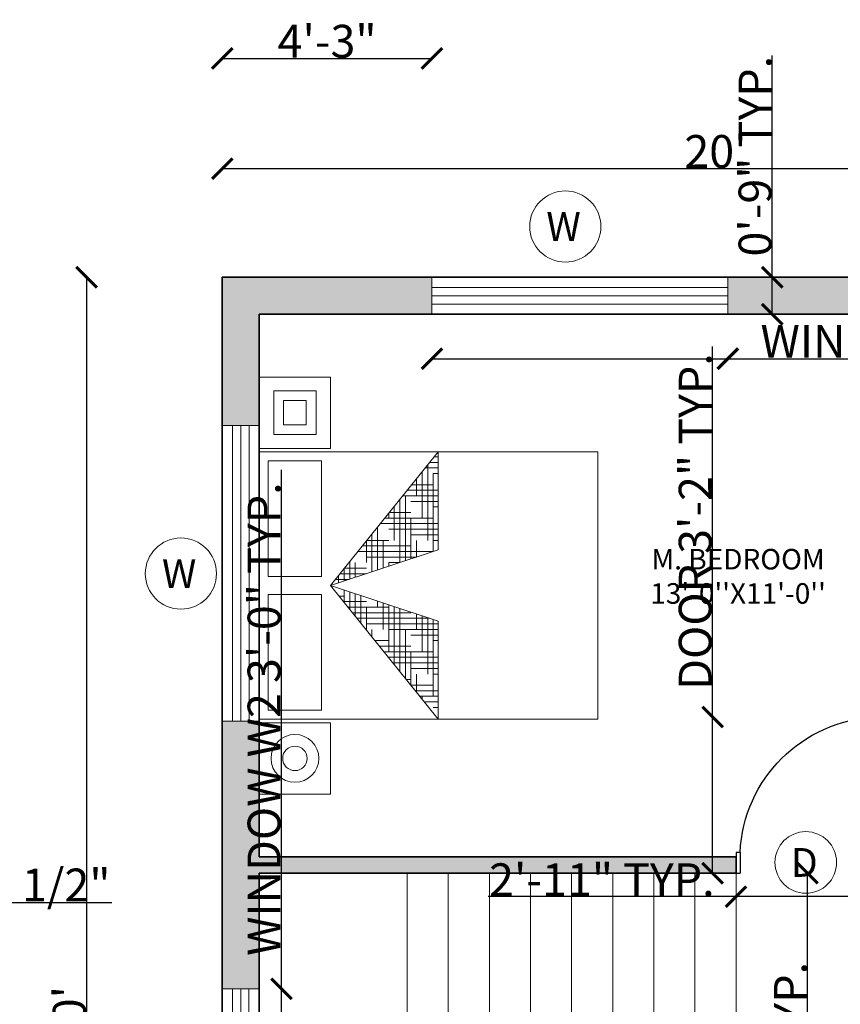
# Model space of a CAD drawing. Units: inches. Extents: x 2209 to 2954, y 1760 to 2265.
# Tile 6 of 7: x 2580 to 2780, y 2005 to 2245. Entities that reach past the tile are written whole.
import ezdxf

# ---------------------------------------------------------------- set-up
doc = ezdxf.new("R2010")
doc.units = ezdxf.units.IN
for name, color, linetype, lineweight in [('A-ANNO-DIMS', 2, 'Continuous', 18), ('A-ANNO-SYMB', 7, 'Continuous', 18), ('A-AREA-IDEN', 7, 'Continuous', 18), ('A-FURN', 8, 'Continuous', 18), ('A-WALL-PATT', 30, 'Continuous', 13), ('DOOR', 240, 'Continuous', 25), ('STEPS', 50, 'Continuous', 18), ('WALL', 7, 'Continuous', 35), ('WINDOW', 190, 'Continuous', 18)]:
    doc.layers.add(name, color=color, linetype=linetype, lineweight=lineweight)
doc.styles.get("Standard").update_dxf_attribs({"font": 'arial.ttf'})
doc.dimstyles.get("Standard").update_dxf_attribs({"dimtxt": 8, "dimasz": 5, "dimexe": 0.18, "dimexo": 0.0625, "dimgap": 0.09, "dimtad": 1, "dimdec": 1, "dimzin": 0, "dimdsep": 46, "dimlunit": 4, "dimtxsty": 'Standard', "dimblk": 'ARCHTICK', "dimcen": 0.09, "dimse1": 1, "dimse2": 1, "dimadec": 0, "dimazin": 0, "dimtfac": 1, "dimtdec": 1, "dimtofl": 0, "dimtmove": 0, "dimatfit": 3, "dimfxl": 1, "dimtolj": 1, "dimtzin": 0, "dimarcsym": 0})

# ---------------------------------------------------------------- blocks, each defined once
blk = doc.blocks.new('AP0B05')
for p, q in [((35, 100), (35, 880)), ((75, 100), (75, 878.9)), ((35, 100), (11, 100)), ((11, 100), (11, -20)), ((35, 100), (35, -20)), ((815, 100), (815, -20)), ((815, 100), (839, 100)), ((839, 100), (839, -20)), ((11, -20), (35, -20)), ((839, -20), (815, -20))]:
    blk.add_line(p, q)
blk.add_lwpolyline([(35, 100), (75, 100)])
blk.add_arc((-2.4, 62.6), 818.3, 2.6212, 87.3788)
blk = doc.blocks.new('*X3')
at = {"color": 0}
for p, q in [((20.25, 14.8125), (20.2772, 14.8125)), ((20.1875, 14.75), (20.1875, 14.7669)), ((20.199, 14.7812), (20.2772, 14.7812)), ((20.1487, 14.7188), (20.2772, 14.7188)), ((20.1562, 14.625), (20.1562, 14.7281)), ((20.1739, 14.75), (20.2772, 14.75)), ((20.25, 14.3194), (20.25, 14.75)), ((20.0938, 14.375), (20.0938, 14.6504)), ((20.0984, 14.6562), (20.125, 14.6562)), ((20.1236, 14.6875), (20.25, 14.6875)), ((20.125, 14.5), (20.125, 14.6893)), ((20.0625, 14.2573), (20.0625, 14.6116)), ((20.125, 14.5938), (20.2772, 14.5938)), ((20.2188, 14.3091), (20.2188, 14.625)), ((20.25, 14.625), (20.2772, 14.625)), ((20.023, 14.5625), (20.2772, 14.5625)), ((20.0312, 14.2469), (20.0312, 14.5727)), ((19.9727, 14.5), (20.25, 14.5)), ((19.9979, 14.5312), (20.2772, 14.5312)), ((20, 14.2366), (20, 14.5)), ((20.1875, 14.2987), (20.1875, 14.5)), ((19.9225, 14.4375), (20, 14.4375)), ((19.9476, 14.4688), (20.125, 14.4688)), ((20.25, 14.4375), (20.2772, 14.4375)), ((19.875, 14.25), (19.875, 14.3785)), ((19.9062, 14.375), (19.9062, 14.4174)), ((19.9688, 14.2262), (19.9688, 14.375)), ((20, 14.375), (20.2772, 14.375)), ((20.125, 14.4062), (20.2772, 14.4062)), ((20.1562, 14.2884), (20.1562, 14.375)), ((19.8219, 14.3125), (20.2291, 14.3125)), ((19.8438, 14.1848), (19.8438, 14.3397)), ((19.875, 14.3438), (20.2772, 14.3438)), ((19.7812, 14.1641), (19.7812, 14.262)), ((19.7967, 14.2812), (20.125, 14.2812)), ((19.8125, 14.1744), (19.8125, 14.3008)), ((19.7465, 14.2188), (19.875, 14.2188)), ((19.75, 14.1537), (19.75, 14.2231)), ((19.7716, 14.25), (20, 14.25)), ((19.9375, 14.2159), (19.9375, 14.25)), ((19.7213, 14.1875), (19.75, 14.1875)), ((19.7018, 14.0938), (19.7786, 14.0938)), ((19.7188, 14.0726), (19.7188, 14.1136)), ((19.75, 14.0338), (19.75, 14.1032)), ((19.7812, 13.9949), (19.7812, 14.0929)), ((19.7269, 14.0625), (19.8728, 14.0625)), ((19.8125, 14), (19.8125, 14.0825)), ((19.9062, 13.8396), (19.9062, 14.0514)), ((19.9375, 13.8007), (19.9375, 14.0411)), ((19.752, 14.0312), (19.875, 14.0312)), ((19.875, 13.8784), (19.875, 14)), ((19.9688, 13.875), (19.9688, 14.0307)), ((20, 14), (20, 14.0204)), ((20, 14), (20.0614, 14)), ((20.0625, 13.6454), (20.0625, 13.9996)), ((20.0938, 13.625), (20.0938, 13.9893)), ((19.8275, 13.9375), (20.25, 13.9375)), ((19.875, 13.9688), (20.1557, 13.9688)), ((20.125, 13.75), (20.125, 13.9789)), ((20.1562, 13.875), (20.1562, 13.9686)), ((20.25, 13.5), (20.25, 13.9375)), ((19.8526, 13.9062), (20.125, 13.9062)), ((19.8777, 13.875), (20, 13.875)), ((20.0312, 13.6842), (20.0312, 13.875)), ((20.2188, 13.4511), (20.2188, 13.875)), ((20.25, 13.875), (20.2772, 13.875)), ((20.125, 13.8438), (20.2772, 13.8438)), ((19.9532, 13.7812), (20.2772, 13.7812)), ((20, 13.8125), (20.2772, 13.8125)), ((19.9783, 13.75), (20.25, 13.75)), ((20, 13.723), (20, 13.75)), ((20.0035, 13.7188), (20.125, 13.7188)), ((20.1875, 13.49), (20.1875, 13.75)), ((20.125, 13.6562), (20.2772, 13.6562)), ((20.25, 13.6875), (20.2772, 13.6875)), ((20.0789, 13.625), (20.2772, 13.625)), ((20.104, 13.5938), (20.2772, 13.5938)), ((20.1562, 13.5288), (20.1562, 13.625)), ((20.1292, 13.5625), (20.25, 13.5625)), ((20.25, 13.5), (20.2772, 13.5)), ((20.2046, 13.4688), (20.2772, 13.4688)), ((20.2297, 13.4375), (20.2772, 13.4375)), ((20.2549, 13.4062), (20.2772, 13.4062))]:
    blk.add_line(p, q, dxfattribs=at)
blk = doc.blocks.new('MAT-P13')
for p, q in [((-1.17, 0), (-1.17, -0.4)), ((-1.17, 0), (-0.77, 0)), ((-0.77, 0), (-0.77, -0.4)), ((-0.75, 0), (0.75, 0)), ((-0.75, 0), (-0.75, -1.9)), ((0.75, 0), (0.75, -1.9)), ((0.77, 0), (1.17, 0)), ((0.77, 0), (0.77, -0.4)), ((1.17, 0), (1.17, -0.4)), ((-0.7, -0.05), (-0.7, -0.35)), ((-0.7, -0.05), (-0.05, -0.05)), ((-0.05, -0.35), (-0.05, -0.05)), ((0.05, -0.05), (0.7, -0.05)), ((0.05, -0.35), (0.05, -0.05)), ((0.7, -0.05), (0.7, -0.35)), ((-0.7, -0.35), (-0.05, -0.35)), ((0.05, -0.35), (0.7, -0.35)), ((-1.17, -0.4), (-0.77, -0.4)), ((-0.75, -1.0034), (0, -0.4)), ((0, -0.4), (-0.75, -1.0034)), ((0, -0.4), (-0.2, -1.0034)), ((0, -0.4), (0.2, -1.0034)), ((0, -0.4), (0.75, -1.0034)), ((0.77, -0.4), (1.17, -0.4)), ((-0.75, -1.0034), (-0.2, -1.0034)), ((0.2, -1.0034), (0.75, -1.0034)), ((0.75, -1.9), (-0.75, -1.9))]:
    blk.add_line(p, q)
for points in [[(0.8468, -0.0814), (1.0932, -0.0814), (1.0932, -0.3186), (0.8468, -0.3186)], [(0.9015, -0.1361), (1.0385, -0.1361), (1.0385, -0.2639), (0.9015, -0.2639)]]:
    blk.add_lwpolyline(points, close=True)
for radius in [0.1342, 0.0686]:
    blk.add_circle((-0.97, -0.2), radius)
at = {"xscale": -1, "rotation": 90}
blk.add_blockref('*X3', (14.1285, 19.2738), dxfattribs=at)
blk = doc.blocks.new('_ArchTick')
at = {"color": 0, "linetype": 'ByBlock', "const_width": 0.15}
blk.add_lwpolyline([(-0.5, -0.5), (0.5, 0.5)], dxfattribs=at)
blk = doc.blocks.new('*D15')
at = {"layer": 'A-ANNO-DIMS', "color": 0, "lineweight": -2, "transparency": 16777216}
blk.add_line((2629.22, 2208.74), (2869.22, 2208.74), dxfattribs=at)
at = {"layer": 'Defpoints', "color": 0, "transparency": 16777216}
for p in [(2869.22, 2208.74), (2629.22, 2182.29), (2869.22, 2182.29)]:
    blk.add_point(p, dxfattribs=at)
at = {"layer": 'A-ANNO-DIMS', "color": 0, "lineweight": -2, "transparency": 16777216, "xscale": 5, "yscale": 5, "zscale": 5, "rotation": 180}
blk.add_blockref('_ArchTick', (2629.22, 2208.74), dxfattribs=at)
at = {"layer": 'A-ANNO-DIMS', "color": 0, "lineweight": -2, "transparency": 16777216, "xscale": 5, "yscale": 5, "zscale": 5}
blk.add_blockref('_ArchTick', (2869.22, 2208.74), dxfattribs=at)
at = {"layer": 'A-ANNO-DIMS', "color": 0, "transparency": 16777216, "insert": (2749.22, 2212.91), "char_height": 8, "attachment_point": 5}
blk.add_mtext("\\A1;20'", dxfattribs=at)
blk = doc.blocks.new('*D16')
at = {"layer": 'A-ANNO-DIMS', "color": 0, "lineweight": -2, "transparency": 16777216}
blk.add_line((2596.18, 2182.29), (2596.18, 1822.29), dxfattribs=at)
at = {"layer": 'Defpoints', "color": 0, "transparency": 16777216}
for p in [(2629.22, 2182.29), (2596.18, 1822.29), (2629.22, 1822.29)]:
    blk.add_point(p, dxfattribs=at)
at = {"layer": 'A-ANNO-DIMS', "color": 0, "lineweight": -2, "transparency": 16777216, "xscale": 5, "yscale": 5, "zscale": 5}
for p, rotation in [((2596.18, 2182.29), 90), ((2596.18, 1822.29), 270)]:
    blk.add_blockref('_ArchTick', p, dxfattribs=dict(at, rotation=rotation))
at = {"layer": 'A-ANNO-DIMS', "color": 0, "transparency": 16777216, "insert": (2592, 2002.29), "char_height": 8, "attachment_point": 5, "rotation": 90}
blk.add_mtext("\\A1;30'", dxfattribs=at)
blk = doc.blocks.new('WIN-W-72IN')
for p, q in [((0, 6.5), (72, 6.5)), ((0, 4.5), (72, 4.5)), ((0, 2.5), (72, 2.5))]:
    blk.add_line(p, q)
blk.add_lwpolyline([(0, 9), (72, 9), (72, 0), (0, 0)], close=True)
blk = doc.blocks.new('WIN-W2-36IN')
for p, q in [((2.5, 0), (2.5, 36)), ((4.5, 0), (4.5, 36)), ((6.5, 0), (6.5, 36))]:
    blk.add_line(p, q)
blk.add_lwpolyline([(0, 0), (0, 36), (9, 36), (9, 0)], close=True)
blk = doc.blocks.new('STAIR-RETURN-36IN')
for p, q in [((36, 0), (36, 92)), ((46, 56), (46, 92)), ((56, 56), (56, 92)), ((66, 56), (66, 92)), ((76, 56), (76, 92)), ((86, 56), (86, 92)), ((96, 56), (96, 92)), ((106, 56), (106, 92)), ((116, 56), (116, 92)), ((116, 56), (0, 56)), ((36, 46), (0, 46)), ((106, 36), (0, 36)), ((46, 0), (46, 36)), ((56, 0), (56, 36)), ((66, 0), (66, 36)), ((76, 0), (76, 36)), ((86, 0), (86, 36)), ((96, 0), (96, 36)), ((106, 0), (106, 36))]:
    blk.add_line(p, q)
blk = doc.blocks.new('TAG-OPENING-W')
blk.add_circle((0, 0), 8.66)
blk.add_text('W', height=7).set_placement((-4.62, -3.5))
blk = doc.blocks.new('TAG-OPENING-D')
blk.add_circle((0, 0), 7.5)
blk.add_text('D', height=7).set_placement((-3.65, -3.5))
blk = doc.blocks.new('*D27')
at = {"layer": 'A-ANNO-DIMS', "color": 0, "lineweight": -2, "transparency": 16777216}
for p, q in [((2680.22, 2162.49), (2752.22, 2162.49)), ((2752.22, 2162.49), (2872.28, 2162.49))]:
    blk.add_line(p, q, dxfattribs=at)
at = {"layer": 'Defpoints', "color": 0, "transparency": 16777216}
for p in [(2680.22, 2173.29), (2752.22, 2173.29), (2752.22, 2162.49)]:
    blk.add_point(p, dxfattribs=at)
at = {"layer": 'A-ANNO-DIMS', "color": 0, "lineweight": -2, "transparency": 16777216, "xscale": 5, "yscale": 5, "zscale": 5, "rotation": 180}
blk.add_blockref('_ArchTick', (2680.22, 2162.49), dxfattribs=at)
at = {"layer": 'A-ANNO-DIMS', "color": 0, "lineweight": -2, "transparency": 16777216, "xscale": 5, "yscale": 5, "zscale": 5}
blk.add_blockref('_ArchTick', (2752.22, 2162.49), dxfattribs=at)
at = {"layer": 'A-ANNO-DIMS', "color": 0, "transparency": 16777216, "insert": (2814.75, 2166.71), "char_height": 8, "attachment_point": 5}
blk.add_mtext('\\A1;WINDOW W 6\'-0" TYP.', dxfattribs=at)
blk = doc.blocks.new('*D28')
at = {"layer": 'A-ANNO-DIMS', "color": 0, "lineweight": -2, "transparency": 16777216}
for p, q in [((2763.02, 2182.29), (2763.02, 2236.23)), ((2763.02, 2173.29), (2763.02, 2182.29))]:
    blk.add_line(p, q, dxfattribs=at)
at = {"layer": 'Defpoints', "color": 0, "transparency": 16777216}
for p in [(2752.22, 2182.29), (2763.02, 2182.29), (2752.22, 2173.29)]:
    blk.add_point(p, dxfattribs=at)
at = {"layer": 'A-ANNO-DIMS', "color": 0, "lineweight": -2, "transparency": 16777216, "xscale": 5, "yscale": 5, "zscale": 5}
for p, rotation in [((2763.02, 2182.29), 90), ((2763.02, 2173.29), 270)]:
    blk.add_blockref('_ArchTick', p, dxfattribs=dict(at, rotation=rotation))
at = {"layer": 'A-ANNO-DIMS', "color": 0, "transparency": 16777216, "insert": (2758.84, 2211.76), "char_height": 8, "attachment_point": 5, "rotation": 90}
blk.add_mtext('\\A1;0\'-9" TYP.', dxfattribs=at)
blk = doc.blocks.new('*D29')
at = {"layer": 'A-ANNO-DIMS', "color": 0, "lineweight": -2, "transparency": 16777216}
for p, q in [((2643.62, 2009.14), (2643.62, 2135.42)), ((2643.62, 1973.14), (2643.62, 2009.14))]:
    blk.add_line(p, q, dxfattribs=at)
at = {"layer": 'Defpoints', "color": 0, "transparency": 16777216}
for p in [(2638.22, 2009.14), (2643.62, 2009.14), (2638.22, 1973.14)]:
    blk.add_point(p, dxfattribs=at)
at = {"layer": 'A-ANNO-DIMS', "color": 0, "lineweight": -2, "transparency": 16777216, "xscale": 5, "yscale": 5, "zscale": 5}
for p, rotation in [((2643.62, 2009.14), 90), ((2643.62, 1973.14), 270)]:
    blk.add_blockref('_ArchTick', p, dxfattribs=dict(at, rotation=rotation))
at = {"layer": 'A-ANNO-DIMS', "color": 0, "transparency": 16777216, "insert": (2639.38, 2074.78), "char_height": 8, "attachment_point": 5, "rotation": 90}
blk.add_mtext('\\A1;WINDOW W2 3\'-0" TYP.', dxfattribs=at)
blk = doc.blocks.new('*D37')
at = {"layer": 'A-ANNO-DIMS', "color": 0, "lineweight": -2, "transparency": 16777216}
for p, q in [((2748.52, 2075.28), (2748.52, 2165.46)), ((2748.52, 2037.29), (2748.52, 2075.28))]:
    blk.add_line(p, q, dxfattribs=at)
at = {"layer": 'Defpoints', "color": 0, "transparency": 16777216}
for p in [(2748.52, 2075.28), (2754.22, 2075.28), (2754.22, 2037.29)]:
    blk.add_point(p, dxfattribs=at)
at = {"layer": 'A-ANNO-DIMS', "color": 0, "lineweight": -2, "transparency": 16777216, "xscale": 5, "yscale": 5, "zscale": 5}
for p, rotation in [((2748.52, 2075.28), 90), ((2748.52, 2037.29), 270)]:
    blk.add_blockref('_ArchTick', p, dxfattribs=dict(at, rotation=rotation))
at = {"layer": 'A-ANNO-DIMS', "color": 0, "transparency": 16777216, "insert": (2744.28, 2122.87), "char_height": 8, "attachment_point": 5, "rotation": 90}
blk.add_mtext('\\A1;DOOR 3\'-2" TYP.', dxfattribs=at)
blk = doc.blocks.new('*D38')
at = {"layer": 'A-ANNO-DIMS', "color": 0, "lineweight": -2, "transparency": 16777216}
for p, q in [((2754.22, 2031.59), (2693.92, 2031.59)), ((2789.17, 2031.59), (2754.22, 2031.59))]:
    blk.add_line(p, q, dxfattribs=at)
at = {"layer": 'Defpoints', "color": 0, "transparency": 16777216}
for p in [(2754.22, 2037.29), (2789.17, 2037.29), (2754.22, 2031.59)]:
    blk.add_point(p, dxfattribs=at)
at = {"layer": 'A-ANNO-DIMS', "color": 0, "lineweight": -2, "transparency": 16777216, "xscale": 5, "yscale": 5, "zscale": 5, "rotation": 180}
blk.add_blockref('_ArchTick', (2754.22, 2031.59), dxfattribs=at)
at = {"layer": 'A-ANNO-DIMS', "color": 0, "lineweight": -2, "transparency": 16777216, "xscale": 5, "yscale": 5, "zscale": 5}
blk.add_blockref('_ArchTick', (2789.17, 2031.59), dxfattribs=at)
at = {"layer": 'A-ANNO-DIMS', "color": 0, "transparency": 16777216, "insert": (2721.57, 2035.7), "char_height": 8, "attachment_point": 5}
blk.add_mtext('\\A1;2\'-11" TYP.', dxfattribs=at)
blk = doc.blocks.new('*D52')
at = {"layer": 'A-ANNO-DIMS', "color": 0, "lineweight": -2, "transparency": 16777216}
blk.add_line((2771.62, 1945.29), (2771.62, 2037.29), dxfattribs=at)
at = {"layer": 'Defpoints', "color": 0, "transparency": 16777216}
for p in [(2754.22, 2037.29), (2771.62, 2037.29), (2754.22, 1945.29)]:
    blk.add_point(p, dxfattribs=at)
at = {"layer": 'A-ANNO-DIMS', "color": 0, "lineweight": -2, "transparency": 16777216, "xscale": 5, "yscale": 5, "zscale": 5}
for p, rotation in [((2771.62, 2037.29), 90), ((2771.62, 1945.29), 270)]:
    blk.add_blockref('_ArchTick', p, dxfattribs=dict(at, rotation=rotation))
at = {"layer": 'A-ANNO-DIMS', "color": 0, "transparency": 16777216, "insert": (2767.44, 1991.29), "char_height": 8, "attachment_point": 5, "rotation": 90}
blk.add_mtext('\\A1;7\'-8" TYP.', dxfattribs=at)
blk = doc.blocks.new('*D61')
at = {"layer": 'A-ANNO-DIMS', "color": 0, "lineweight": -2, "transparency": 16777216}
for p, q in [((2429.48, 2030.19), (2506.77, 2030.19)), ((2506.77, 2030.19), (2602.37, 2030.19))]:
    blk.add_line(p, q, dxfattribs=at)
at = {"layer": 'Defpoints', "color": 0, "transparency": 16777216}
for p in [(2506.77, 2030.19), (2429.48, 2018.6), (2506.77, 2018.6)]:
    blk.add_point(p, dxfattribs=at)
at = {"layer": 'A-ANNO-DIMS', "color": 0, "lineweight": -2, "transparency": 16777216, "xscale": 5, "yscale": 5, "zscale": 5, "rotation": 180}
blk.add_blockref('_ArchTick', (2429.48, 2030.19), dxfattribs=at)
at = {"layer": 'A-ANNO-DIMS', "color": 0, "lineweight": -2, "transparency": 16777216, "xscale": 5, "yscale": 5, "zscale": 5}
blk.add_blockref('_ArchTick', (2506.77, 2030.19), dxfattribs=at)
at = {"layer": 'A-ANNO-DIMS', "color": 0, "transparency": 16777216, "insert": (2557.07, 2034.42), "char_height": 8, "attachment_point": 5}
blk.add_mtext('\\A1;DINETTE 6\'-5 1/2"', dxfattribs=at)
blk = doc.blocks.new('*D76')
at = {"layer": 'A-ANNO-DIMS', "color": 0, "lineweight": -2, "transparency": 16777216}
for p, q in [((2920.04, 2077.63), (2920.04, 2129.07)), ((2920.04, 2043.25), (2920.04, 2077.63))]:
    blk.add_line(p, q, dxfattribs=at)
at = {"layer": 'Defpoints', "color": 0, "transparency": 16777216}
for p in [(2519.15, 2077.63), (2920.04, 2077.63), (2519.15, 2043.25)]:
    blk.add_point(p, dxfattribs=at)
at = {"layer": 'A-ANNO-DIMS', "color": 0, "lineweight": -2, "transparency": 16777216, "xscale": 5, "yscale": 5, "zscale": 5}
for p, rotation in [((2920.04, 2077.63), 90), ((2920.04, 2043.25), 270)]:
    blk.add_blockref('_ArchTick', p, dxfattribs=dict(at, rotation=rotation))
at = {"layer": 'A-ANNO-DIMS', "color": 0, "transparency": 16777216, "insert": (2915.82, 2105.85), "char_height": 8, "attachment_point": 5, "rotation": 90}
blk.add_mtext('\\A1;2\'-10 1/2"', dxfattribs=at)
blk = doc.blocks.new('*D77')
at = {"layer": 'A-ANNO-DIMS', "color": 0, "lineweight": -2, "transparency": 16777216}
for p, q in [((2920.04, 2131.29), (2920.04, 2175.62)), ((2920.04, 2113.63), (2920.04, 2131.29))]:
    blk.add_line(p, q, dxfattribs=at)
at = {"layer": 'Defpoints', "color": 0, "transparency": 16777216}
for p in [(2519.15, 2131.29), (2920.04, 2131.29), (2519.15, 2113.63)]:
    blk.add_point(p, dxfattribs=at)
at = {"layer": 'A-ANNO-DIMS', "color": 0, "lineweight": -2, "transparency": 16777216, "xscale": 5, "yscale": 5, "zscale": 5}
for p, rotation in [((2920.04, 2131.29), 90), ((2920.04, 2113.63), 270)]:
    blk.add_blockref('_ArchTick', p, dxfattribs=dict(at, rotation=rotation))
at = {"layer": 'A-ANNO-DIMS', "color": 0, "transparency": 16777216, "insert": (2915.82, 2155.95), "char_height": 8, "attachment_point": 5, "rotation": 90}
blk.add_mtext('\\A1;1\'-5 1/2"', dxfattribs=at)
blk = doc.blocks.new('*D86')
at = {"layer": 'A-ANNO-DIMS', "color": 0, "lineweight": -2, "transparency": 16777216}
blk.add_line((2629.22, 2235.55), (2680.22, 2235.55), dxfattribs=at)
at = {"layer": 'Defpoints', "color": 0, "transparency": 16777216}
for p in [(2680.22, 2235.55), (2629.22, 2182.29), (2680.22, 2182.29)]:
    blk.add_point(p, dxfattribs=at)
at = {"layer": 'A-ANNO-DIMS', "color": 0, "lineweight": -2, "transparency": 16777216, "xscale": 5, "yscale": 5, "zscale": 5, "rotation": 180}
blk.add_blockref('_ArchTick', (2629.22, 2235.55), dxfattribs=at)
at = {"layer": 'A-ANNO-DIMS', "color": 0, "lineweight": -2, "transparency": 16777216, "xscale": 5, "yscale": 5, "zscale": 5}
blk.add_blockref('_ArchTick', (2680.22, 2235.55), dxfattribs=at)
at = {"layer": 'A-ANNO-DIMS', "color": 0, "transparency": 16777216, "insert": (2654.72, 2239.73), "char_height": 8, "attachment_point": 5}
blk.add_mtext('\\A1;4\'-3"', dxfattribs=at)
blk = doc.blocks.new('*D87')
at = {"layer": 'A-ANNO-DIMS', "color": 0, "lineweight": -2, "transparency": 16777216}
blk.add_line((2224.78, 2146.27), (2224.78, 2182.29), dxfattribs=at)
at = {"layer": 'Defpoints', "color": 0, "transparency": 16777216}
for p in [(2224.78, 2182.29), (2629.22, 2182.29), (2629.22, 2146.27)]:
    blk.add_point(p, dxfattribs=at)
at = {"layer": 'A-ANNO-DIMS', "color": 0, "lineweight": -2, "transparency": 16777216, "xscale": 5, "yscale": 5, "zscale": 5}
for p, rotation in [((2224.78, 2182.29), 90), ((2224.78, 2146.27), 270)]:
    blk.add_blockref('_ArchTick', p, dxfattribs=dict(at, rotation=rotation))
at = {"layer": 'A-ANNO-DIMS', "color": 0, "transparency": 16777216, "insert": (2220.6, 2164.28), "char_height": 8, "attachment_point": 5, "rotation": 90}
blk.add_mtext('\\A1;3\'-0"', dxfattribs=at)
blk = doc.blocks.new('*D89')
at = {"layer": 'A-ANNO-DIMS', "color": 0, "lineweight": -2, "transparency": 16777216}
blk.add_line((2224.78, 2009.14), (2224.78, 2074.27), dxfattribs=at)
at = {"layer": 'Defpoints', "color": 0, "transparency": 16777216}
for p in [(2224.78, 2074.27), (2629.22, 2074.27), (2629.22, 2009.14)]:
    blk.add_point(p, dxfattribs=at)
at = {"layer": 'A-ANNO-DIMS', "color": 0, "lineweight": -2, "transparency": 16777216, "xscale": 5, "yscale": 5, "zscale": 5}
for p, rotation in [((2224.78, 2074.27), 90), ((2224.78, 2009.14), 270)]:
    blk.add_blockref('_ArchTick', p, dxfattribs=dict(at, rotation=rotation))
at = {"layer": 'A-ANNO-DIMS', "color": 0, "transparency": 16777216, "insert": (2220.62, 2041.7), "char_height": 8, "attachment_point": 5, "rotation": 90}
blk.add_mtext('\\A1;5\'-5"', dxfattribs=at)
blk = doc.blocks.new('*D93')
at = {"layer": 'A-ANNO-DIMS', "color": 0, "lineweight": -2, "transparency": 16777216}
for p, q in [((2224.78, 2107.29), (2224.78, 2133.73)), ((2224.78, 2103.29), (2224.78, 2107.29))]:
    blk.add_line(p, q, dxfattribs=at)
at = {"layer": 'Defpoints', "color": 0, "transparency": 16777216}
for p in [(2224.78, 2107.29), (2798.22, 2107.29), (2798.22, 2103.29)]:
    blk.add_point(p, dxfattribs=at)
at = {"layer": 'A-ANNO-DIMS', "color": 0, "lineweight": -2, "transparency": 16777216, "xscale": 5, "yscale": 5, "zscale": 5}
for p, rotation in [((2224.78, 2107.29), 90), ((2224.78, 2103.29), 270)]:
    blk.add_blockref('_ArchTick', p, dxfattribs=dict(at, rotation=rotation))
at = {"layer": 'A-ANNO-DIMS', "color": 0, "transparency": 16777216, "insert": (2220.61, 2123.01), "char_height": 8, "attachment_point": 5, "rotation": 90}
blk.add_mtext('\\A1;0\'-4"', dxfattribs=at)

msp = doc.modelspace()

# ---------------------------------------------------------------- hatches: boundary and pattern name
at = {"layer": 'A-WALL-PATT', "transparency": 33554585}
h = msp.add_hatch(color=256, dxfattribs=at)
h.dxf.hatch_style = 1
h.paths.add_polyline_path([(2519.15, 2182.29), (2402.15, 2182.29), (2402.15, 2173.29), (2444.15, 2173.29), (2444.15, 2154.12), (2448.15, 2154.12), (2448.15, 2173.29), (2510.15, 2173.29), (2510.15, 2167.29), (2519.15, 2167.29)])
h.paths.add_polyline_path([(2330.15, 2182.29), (2279.15, 2182.29), (2279.15, 2145.83), (2288.15, 2145.83), (2288.15, 2158.01), (2288.15, 2173.29), (2330.15, 2173.29)])
h.paths.add_polyline_path([(2288.15, 2073.83), (2279.15, 2073.83), (2279.15, 2009.29), (2288.15, 2009.29), (2288.15, 2037.29), (2404.15, 2037.29), (2404.15, 2041.29), (2288.15, 2041.29)])
h.paths.add_polyline_path([(2519.15, 2131.29), (2510.15, 2131.29), (2510.15, 2125.29), (2444.15, 2125.29), (2444.15, 2041.29), (2439.11, 2041.29), (2439.11, 2037.29), (2448.15, 2037.29), (2448.15, 2069.29), (2481.65, 2069.29), (2481.65, 2073.29), (2448.15, 2073.29), (2448.15, 2121.29), (2468.19, 2121.29), (2468.19, 2121.32), (2488.37, 2121.32), (2510.15, 2121.29), (2510.15, 2113.63), (2519.15, 2113.63)])
h.paths.add_polyline_path([(2519.15, 2077.63), (2510.15, 2077.63), (2510.15, 2073.32), (2510.17, 2073.32), (2510.15, 2069.19), (2510.15, 2043.25), (2519.15, 2043.25)], flags=17)
h.paths.add_polyline_path([(2519.15, 1971.25), (2510.15, 1971.25), (2510.15, 1945.29), (2444.15, 1945.29), (2444.15, 1937.21), (2448.15, 1937.21), (2448.15, 1941.29), (2510.15, 1941.29), (2510.15, 1922.29), (2519.15, 1922.29)])
h.paths.add_polyline_path([(2288.15, 1941.29), (2394.15, 1941.29), (2394.15, 1945.29), (2288.15, 1945.29), (2288.15, 1973.29), (2279.15, 1973.29), (2279.15, 1919.97), (2288.15, 1919.97)])
h.paths.add_polyline_path([(2300.65, 1831.29), (2288.15, 1831.29), (2288.15, 1847.97), (2279.15, 1847.97), (2279.15, 1822.29), (2300.65, 1822.29)])
h.paths.add_polyline_path([(2394.15, 1825.29), (2394.15, 1831.29), (2372.65, 1831.29), (2372.65, 1822.29), (2394.15, 1822.29)])
h.paths.add_polyline_path([(2449.17, 1831.29), (2448.15, 1831.29), (2448.15, 1899.32), (2444.15, 1899.32), (2444.15, 1831.29), (2439.18, 1831.29), (2439.18, 1822.29), (2449.17, 1822.29)])
h.paths.add_polyline_path([(2519.15, 1850.29), (2510.15, 1850.29), (2510.15, 1831.29), (2509.17, 1831.29), (2509.17, 1822.29), (2519.15, 1822.29)])
h.paths.add_polyline_path([(2638.22, 1941.29), (2744.22, 1941.29), (2744.22, 1945.29), (2638.22, 1945.29), (2638.22, 1973.14), (2629.22, 1973.14), (2629.22, 1919.53), (2638.22, 1919.53)])
h.paths.add_polyline_path([(2638.22, 1847.53), (2629.22, 1847.53), (2629.22, 1822.29), (2650.72, 1822.29), (2650.72, 1831.29), (2638.22, 1831.29)])
h.paths.add_polyline_path([(2638.22, 2037.29), (2754.22, 2037.29), (2754.22, 2041.29), (2638.22, 2041.29), (2638.22, 2074.27), (2629.22, 2074.27), (2629.22, 2009.14), (2638.22, 2009.14)])
h.paths.add_polyline_path([(2803.22, 1936.29), (2812.78, 1936.29), (2812.78, 1945.29), (2791.22, 1945.29), (2791.22, 1936.29), (2794.22, 1936.29), (2794.22, 1831.29), (2722.72, 1831.29), (2722.72, 1822.29), (2803.22, 1822.29)])
h.paths.add_polyline_path([(2869.22, 1955.43), (2860.22, 1955.43), (2860.22, 1945.29), (2853.36, 1945.29), (2853.36, 1936.29), (2869.22, 1936.29)])
h.paths.add_polyline_path([(2680.22, 2182.29), (2629.22, 2182.29), (2629.22, 2146.27), (2638.22, 2146.27), (2638.22, 2173.29), (2680.22, 2173.29)])
h.paths.add_polyline_path([(2869.22, 2182.29), (2752.22, 2182.29), (2752.22, 2173.29), (2794.22, 2173.29), (2794.22, 2142.92), (2798.22, 2142.92), (2798.22, 2173.29), (2860.22, 2173.29), (2860.22, 2158.46), (2869.22, 2158.46)])
h.paths.add_polyline_path([(2869.22, 2122.46), (2860.22, 2122.46), (2860.22, 2090.29), (2869.22, 2090.29)])

# ---------------------------------------------------------------- linework, layer by layer
at = {"layer": 'WALL'}
for p, q in [((2629.22, 2182.29), (2869.22, 2182.29)), ((2629.22, 2182.29), (2629.22, 1822.29)), ((2638.22, 2173.29), (2794.22, 2173.29)), ((2638.22, 2173.29), (2638.22, 2041.29)), ((2638.22, 2041.29), (2754.22, 2041.29)), ((2754.22, 2037.29), (2754.22, 2041.29)), ((2638.22, 2037.29), (2754.22, 2037.29)), ((2638.22, 2037.29), (2638.22, 1945.29))]:
    msp.add_line(p, q, dxfattribs=at)

# ---------------------------------------------------------------- block references
at = {"layer": 'A-ANNO-SYMB'}
for name, p in [('TAG-OPENING-W', (2712.68, 2194.65)), ('TAG-OPENING-W', (2619.15, 2110.2)), ('TAG-OPENING-D', (2771.19, 2039.91))]:
    msp.add_blockref(name, p, dxfattribs=at)
at = {"layer": 'A-FURN', "xscale": 43.35755422729858, "yscale": 43.35755422729858, "zscale": 43.35755422729858, "rotation": 90}
msp.add_blockref('MAT-P13', (2638.22, 2107.29), dxfattribs=at)
at = {"layer": 'DOOR', "xscale": -0.0422149343000152, "yscale": 0.0422149343000152, "zscale": 0.0422149343000152}
msp.add_blockref('AP0B05', (2789.63, 2038.13), dxfattribs=at)
at = {"layer": 'STEPS'}
msp.add_blockref('STAIR-RETURN-36IN', (2638.21, 1945.29), dxfattribs=at)
at = {"layer": 'WINDOW'}
for name, p in [('WIN-W-72IN', (2680.21, 2173.29)), ('WIN-W2-36IN', (2629.21, 1973.14))]:
    msp.add_blockref(name, p, dxfattribs=at)
at = {"layer": 'WINDOW', "rotation": 89.99999999999984}
msp.add_blockref('WIN-W-72IN', (2638.22, 2074.27), dxfattribs=at)

# ---------------------------------------------------------------- texts
at = {"layer": 'A-AREA-IDEN', "insert": (2732.14, 2116.2), "char_height": 5, "attachment_point": 1}
msp.add_mtext_dynamic_manual_height_columns("\\pxqc;M. BEDROOM\\P13'-0''X11'-0''", width=45.1409, gutter_width=12.5, heights=[0], dxfattribs=at)

# ---------------------------------------------------------------- dimensions: what is measured, and where the dimension line sits
at = {"layer": 'A-ANNO-DIMS'}
for base, p2, override, picture, middle in [((2680.22, 2235.55), (2680.22, 2182.29), {"dimdec": 1, "dimlfac": 1, "dimrnd": 0, "dimzin": 1, "dimdsep": 46, "dimlunit": 4, "dimfrac": 2}, '*D86', (2654.72, 2239.73)), ((2869.22, 2208.74), (2869.22, 2182.29), {"dimclrd": 0, "dimclre": 0, "dimclrt": 0}, '*D15', (2749.22, 2212.91))]:
    dim = msp.add_linear_dim(base=base, p1=(2629.22, 2182.29), p2=p2, dimstyle='Standard', override=override, dxfattribs=at)
    dim.commit()
    dim.dimension.update_dxf_attribs({"geometry": picture, "text_midpoint": middle})
for base, p1, p2, angle, text, picture, middle in [((2763.02, 2182.29), (2752.22, 2173.29), (2752.22, 2182.29), 90, '<> TYP.', '*D28', (2758.84, 2211.76)), ((2748.52, 2075.28), (2754.22, 2037.29), (2754.22, 2075.28), 90, 'DOOR <> TYP.', '*D37', (2744.28, 2122.87)), ((2643.62, 2009.14), (2638.22, 1973.14), (2638.22, 2009.14), 90, 'WINDOW W2 <> TYP.', '*D29', (2639.38, 2074.78)), ((2754.2151, 2031.5861), (2789.1691, 2037.2851), (2754.2151, 2037.2851), 180, '<> TYP.', '*D38', (2721.5672, 2035.6952)), ((2771.62, 2037.29), (2754.22, 1945.29), (2754.22, 2037.29), 90, '<> TYP.', '*D52', (2767.44, 1991.29))]:
    dim = msp.add_linear_dim(base=base, p1=p1, p2=p2, angle=angle, text=text, dimstyle='Standard', override={"dimdec": 1, "dimlfac": 1, "dimrnd": 0, "dimzin": 1, "dimdsep": 46, "dimlunit": 4, "dimfrac": 2}, dxfattribs=at)
    dim.commit()
    dim.dimension.update_dxf_attribs({"geometry": picture, "text_midpoint": middle})
for base, p1, p2, text, picture, middle in [((2752.22, 2162.49), (2680.22, 2173.29), (2752.22, 2173.29), 'WINDOW W <> TYP.', '*D27', (2814.75, 2166.71)), ((2506.77, 2030.19), (2429.48, 2018.6), (2506.77, 2018.6), 'DINETTE <>', '*D61', (2557.07, 2034.42))]:
    dim = msp.add_linear_dim(base=base, p1=p1, p2=p2, text=text, dimstyle='Standard', override={"dimdec": 1, "dimlfac": 1, "dimrnd": 0, "dimzin": 1, "dimdsep": 46, "dimlunit": 4, "dimfrac": 2}, dxfattribs=at)
    dim.commit()
    dim.dimension.update_dxf_attribs({"geometry": picture, "text_midpoint": middle})
for base, p1, p2, override, picture, middle in [((2224.78, 2182.29), (2629.22, 2146.27), (2629.22, 2182.29), {"dimdec": 1, "dimlfac": 1, "dimrnd": 0, "dimzin": 1, "dimdsep": 46, "dimlunit": 4, "dimfrac": 2}, '*D87', (2220.6, 2164.28)), ((2596.18, 1822.29), (2629.22, 2182.29), (2629.22, 1822.29), {"dimclrd": 0, "dimclre": 0, "dimclrt": 0}, '*D16', (2592, 2002.29)), ((2920.04, 2131.29), (2519.15, 2113.63), (2519.15, 2131.29), {"dimdec": 1, "dimlfac": 1, "dimrnd": 0, "dimzin": 1, "dimdsep": 46, "dimlunit": 4, "dimfrac": 2}, '*D77', (2915.82, 2155.95)), ((2224.78, 2107.29), (2798.22, 2103.29), (2798.22, 2107.29), {"dimdec": 1, "dimlfac": 1, "dimrnd": 0, "dimzin": 1, "dimdsep": 46, "dimlunit": 4, "dimfrac": 2}, '*D93', (2220.61, 2123.01)), ((2920.04, 2077.63), (2519.15, 2043.25), (2519.15, 2077.63), {"dimdec": 1, "dimlfac": 1, "dimrnd": 0, "dimzin": 1, "dimdsep": 46, "dimlunit": 4, "dimfrac": 2}, '*D76', (2915.82, 2105.85)), ((2224.78, 2074.27), (2629.22, 2009.14), (2629.22, 2074.27), {"dimdec": 1, "dimlfac": 1, "dimrnd": 0, "dimzin": 1, "dimdsep": 46, "dimlunit": 4, "dimfrac": 2}, '*D89', (2220.62, 2041.7))]:
    dim = msp.add_linear_dim(base=base, p1=p1, p2=p2, angle=90, dimstyle='Standard', override=override, dxfattribs=at)
    dim.commit()
    dim.dimension.update_dxf_attribs({"geometry": picture, "text_midpoint": middle})

doc.saveas('drawing.dxf')
